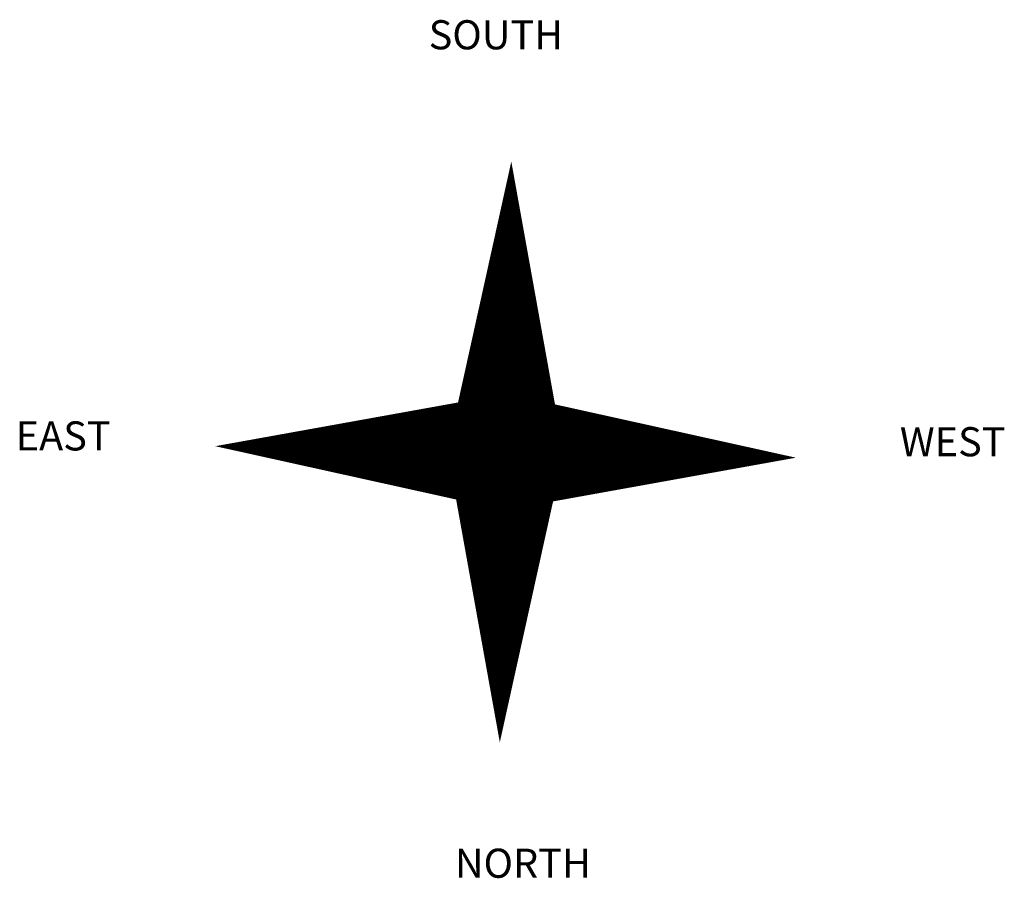
# Model space of a CAD drawing. Units: inches. Extents: x -51 to 1118, y -44 to 791.
# Tile 8 of 8: x 712 to 1118, y 152 to 506. Entities that reach past the tile are written whole.
import ezdxf

# ---------------------------------------------------------------- set-up
doc = ezdxf.new("R2010")
doc.units = ezdxf.units.IN
doc.header["$MEASUREMENT"] = 0
doc.layers.add('A-ANNO-SYMB', color=7, linetype='Continuous', lineweight=25)
doc.styles.get("Standard").update_dxf_attribs({"font": 'arial.ttf'})

msp = doc.modelspace()

# ---------------------------------------------------------------- linework, layer by layer
at = {"layer": 'A-ANNO-SYMB'}
for points in [[(912.15, 327.92, 48, 0, 0), (914.52, 447.62, 0, 0, 0)], [(912.15, 327.92, 48, 0, 0), (792.45, 330.29, 0, 0, 0)], [(912.15, 327.92, 48, 0, 0), (909.78, 208.23, 0, 0, 0)], [(912.15, 327.92, 48, 0, 0), (909.78, 208.23, 0, 0, 0)], [(912.15, 327.92, 48, 0, 0), (1031.84, 325.55, 0, 0, 0)]]:
    msp.add_lwpolyline(points, format="xyseb", dxfattribs=at)

# ---------------------------------------------------------------- texts
for s, p in [('SOUTH', (880.45, 493.83)), ('EAST', (710.21, 328.52)), ('WEST', (1074.67, 326.13)), ('NORTH', (891.24, 152.43))]:
    msp.add_text(s, height=12, dxfattribs=at).set_placement(p)

doc.saveas('drawing.dxf')
